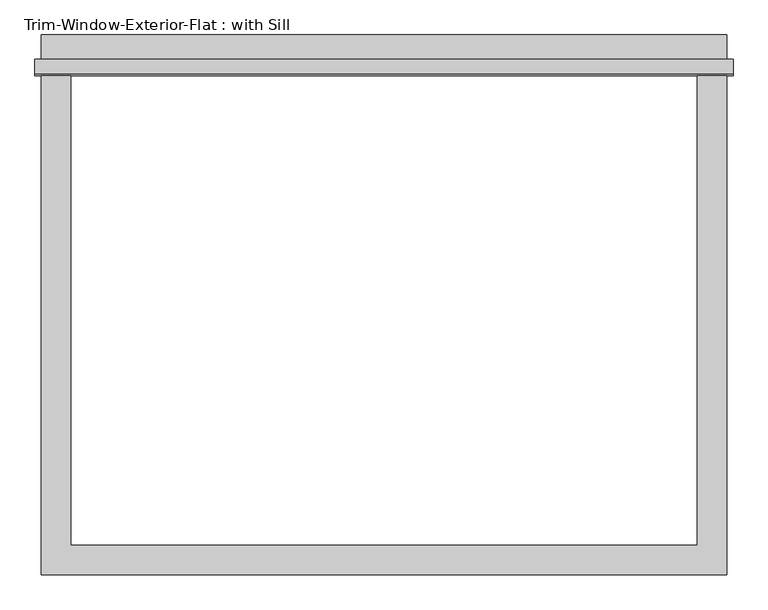
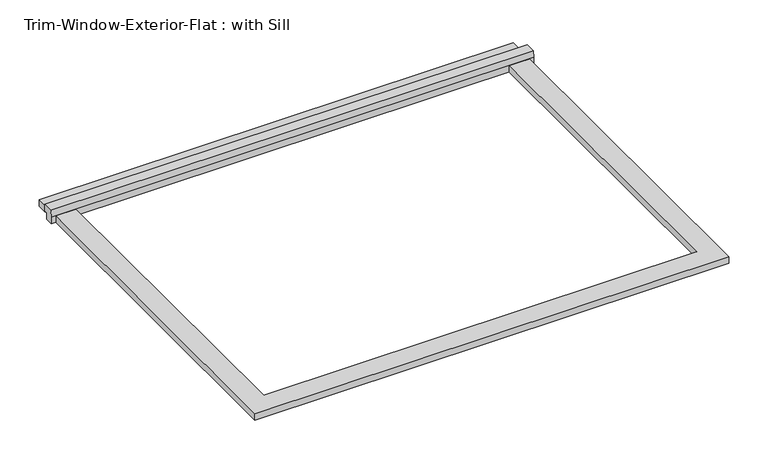
"""IFC4 building model written with IfcOpenShell, lengths in millimetres: proxy geometry, Trim-Window-Exterior-Flat : with Sill."""

from ifc_helpers import new_model, si_unit, frame, origin, origin_with_axes, place, context, project, spatial, polyline, outline, extrude, source, transform, mapped, element, save


def trim_window_exterior_flat_with_sill_729ce974(model_context):
    return source(origin(), model_context, "Body", "SweptSolid", [
        extrude(outline(polyline([(666.75, 936.5823709), (-666.75, 936.5823709), (-666.75, 993.7323709), (666.75, 993.7323709), (666.75, 936.5823709)])), origin_with_axes(), (0.0, 0.0, 1.0), 19.05),
        extrude(outline(polyline([(946.15, 38.1), (946.15, 19.05), (936.5823709, 19.05), (936.5823709, 0.0), (914.4, 0.0), (914.4, 19.05), (916.8580645, 38.1), (946.15, 38.1)])), frame((-679.45, 0.0, 0.0), z_axis=(1.0, 0.0, 0.0), x_axis=(0.0, 1.0, 0.0)), (0.0, 0.0, 1.0), 1358.9),
        extrude(outline(polyline([(-666.75, -57.15), (-666.75, 914.4), (-609.6, 914.4), (-609.6, 0.0), (609.6, 0.0), (609.6, 914.4), (666.75, 914.4), (666.75, -57.15), (-666.75, -57.15)])), origin_with_axes(), (0.0, 0.0, 1.0), 19.05),
    ])


if __name__ == "__main__":
    model = new_model("IFC4")
    model_context = context("Model", 3, world=origin())
    ifc_project = project(units=[si_unit("LENGTHUNIT", "METRE", prefix="MILLI")], contexts=[model_context])
    site = spatial("IfcSite", under=ifc_project)
    building = spatial("IfcBuilding", under=site)
    placement = place(None, origin())
    trim_window_exterior_flat_with_sill_shape = trim_window_exterior_flat_with_sill_729ce974(model_context)
    element("IfcBuildingElementProxy", 1, Name="Trim-Window-Exterior-Flat : with Sill", ObjectType="Trim-Window-Exterior-Flat : with Sill", at=placement, inside=building, context=model_context, shape_type="MappedRepresentation", body=[
        mapped(trim_window_exterior_flat_with_sill_shape, transform((0.0, 0.0, 0.0), x_axis=(1.0, 0.0, 0.0), y_axis=(0.0, 1.0, 0.0), z_axis=(0.0, 0.0, 1.0))),
    ])
    save(model, "model.ifc")

# Revit data of these elements
# Type "Trim-Window-Exterior-Flat : with Sill"
#   Trim Width = 0' - 2 1/4"
#   Trim Thickness_Picture Frame = 0' - 1 1/4"
#   Trim Thickness_with Sill = 0' - 0 3/4"
#   Sill Thickness = 0' - 1 1/4"
#   Opening Width [instance default] = 2' - 0"
#   Opening Height [instance default] = 3' - 0"
#   Default Elevation = 4' - 0"
#   Sill = yes
#   Picture Frame = no
#   Trim Material [instance default] = none
# Element 1 (IfcBuildingElementProxy, "Trim-Window-Exterior-Flat : with Sill")
#   Opening Width = 4' - 0"
#   Trim Material = Clad - White
#   Materials on its faces: "Clad - White"
# Materials
#   "Clad - White": class "Wood", colour RGB 242 242 238, transparency 0, Cost = 0
